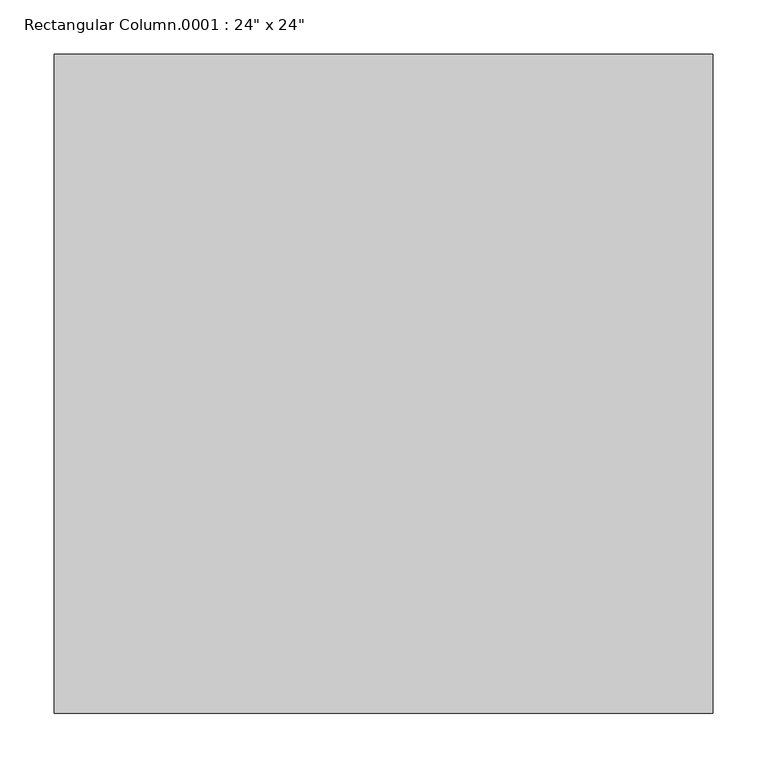
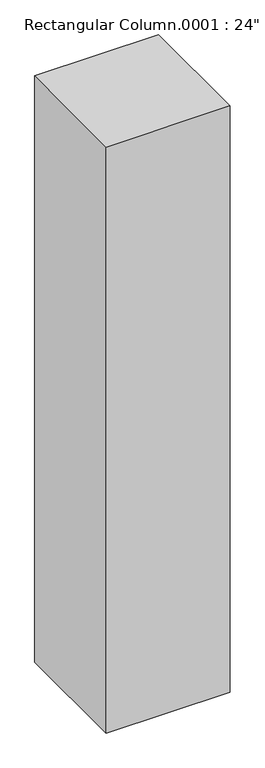
"""IFC4 building model written with IfcOpenShell, lengths in millimetres: column geometry."""

from ifc_helpers import new_model, si_unit, origin, origin_with_axes, place, context, project, spatial, polyline, outline, extrude, source, transform, mapped, element, save


def column_c091e905(model_context):
    return source(origin(), model_context, "Body", "SweptSolid", [
        extrude(outline(polyline([(304.8, 304.8), (304.8, -304.8), (-304.8, -304.8), (-304.8, 304.8), (304.8, 304.8)])), origin_with_axes(), (0.0, 0.0, 1.0), 3048.0),
    ])


if __name__ == "__main__":
    model = new_model("IFC4")
    model_context = context("Model", 3, world=origin())
    ifc_project = project(units=[si_unit("LENGTHUNIT", "METRE", prefix="MILLI")], contexts=[model_context])
    site = spatial("IfcSite", under=ifc_project)
    building = spatial("IfcBuilding", under=site)
    placement = place(None, origin())
    column_shape = column_c091e905(model_context)
    element("IfcColumn", 1, ObjectType="Rectangular Column.0001 : 24\" x 24\"", at=placement, inside=building, context=model_context, shape_type="MappedRepresentation", body=[
        mapped(column_shape, transform((0.0, 0.0, 0.0), x_axis=(1.0, 0.0, 0.0), y_axis=(0.0, 1.0, 0.0), z_axis=(0.0, 0.0, 1.0))),
    ])
    save(model, "model.ifc")

# Revit data of these elements
# Type "Rectangular Column.0001 : 24\" x 24\""
#   Assembly Code = "B1010200"
#   Depth = 2' - 0"
#   Offset Base = 0' - 0"
#   Offset Top = 0' - 0"
#   Width = 2' - 0"
#   Material = Metal - Painted - Grey
# Element 1 (IfcColumn, "Rectangular Column.0001 : 24\" x 24\"")
#   Materials on its faces: "Metal - Painted - Grey"
# Materials
#   "Metal - Painted - Grey": class "Paint", colour RGB 104 104 104, transparency 0, Cost = 0
